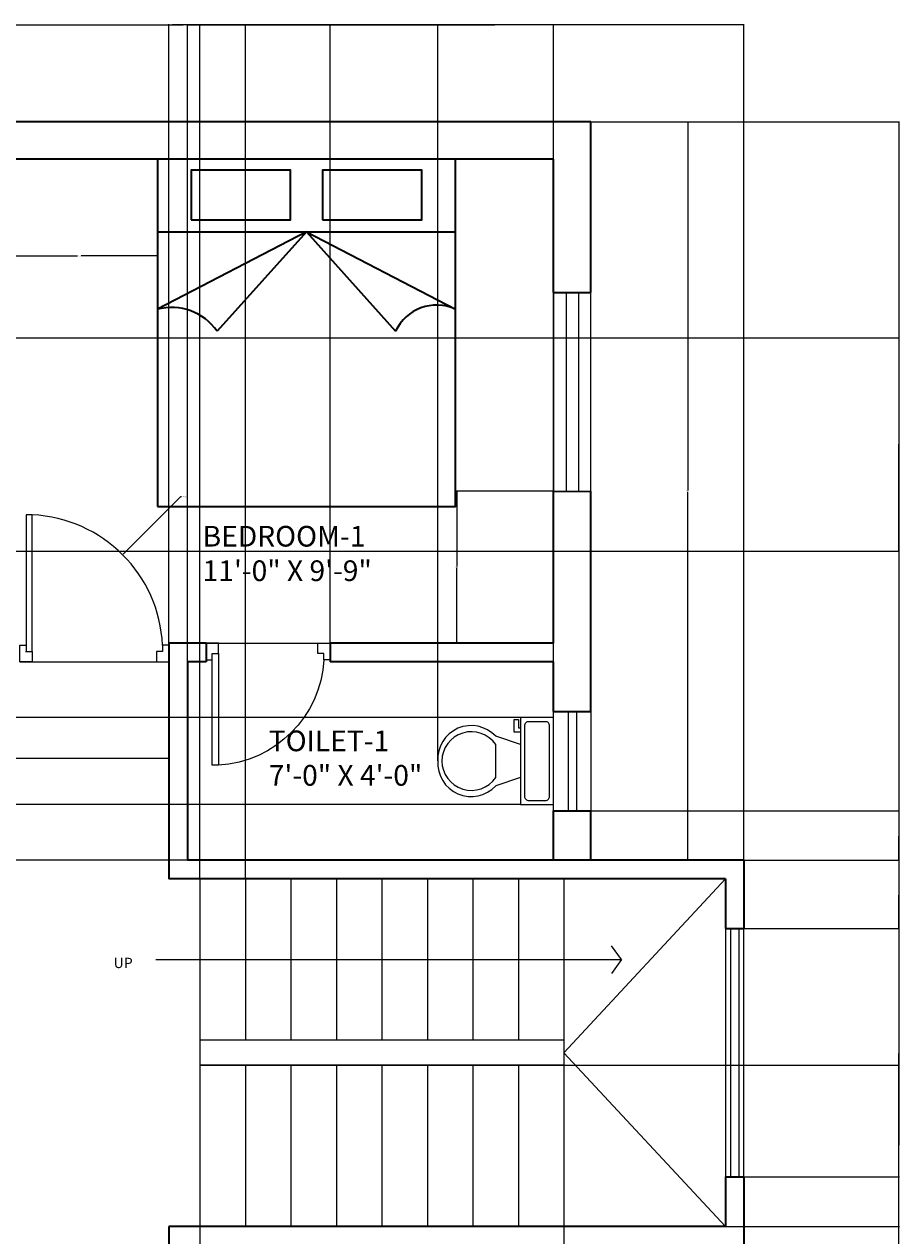
# Model space of a CAD drawing. Units: inches. Extents: x 324 to 662, y 102 to 605.
# Tile 4 of 4: x 451 to 662, y 313 to 605. Entities that reach past the tile are written whole.
import ezdxf

# ---------------------------------------------------------------- set-up
doc = ezdxf.new("R2010")
doc.units = ezdxf.units.IN
for name, color, linetype, lineweight in [('A-ANNO-DIMS', 2, 'Continuous', 18), ('A-ANNO-SYMB', 7, 'Continuous', 18), ('A-ANNO-TEXT', 7, 'Continuous', 18), ('A-AREA-IDEN', 7, 'Continuous', 25), ('A-FLOR-FIXT', 8, 'Continuous', 18), ('A-FLOR-STRS', 7, 'Continuous', 18), ('door', 82, 'Continuous', 25), ('furniture', 8, 'Continuous', 18), ('ventilator', 20, 'Continuous', 18), ('wall', 7, 'Continuous', 35), ('window', 50, 'Continuous', 18)]:
    doc.layers.add(name, color=color, linetype=linetype, lineweight=lineweight)
doc.styles.get("Standard").update_dxf_attribs({"font": 'arial.ttf'})
doc.dimstyles.get("Standard").update_dxf_attribs({"dimtxt": 0.18, "dimasz": 0.18, "dimexe": 0.18, "dimexo": 0.0625, "dimgap": 0.09, "dimtad": 0, "dimtih": 1, "dimtoh": 1, "dimdec": 4, "dimzin": 0, "dimdsep": 46, "dimtxsty": 'Standard', "dimcen": 0.09, "dimadec": 0, "dimazin": 0, "dimtfac": 1, "dimtdec": 4, "dimtofl": 0, "dimtmove": 0, "dimatfit": 3, "dimfxl": 1, "dimtolj": 1, "dimtzin": 0, "dimarcsym": 0})

# ---------------------------------------------------------------- blocks, each defined once
blk = doc.blocks.new('w1')
at = {"layer": 'window'}
for p, q in [((719.66, 290.3), (719.66, 242.3)), ((722.66, 290.3), (722.66, 242.3))]:
    blk.add_line(p, q, dxfattribs=at)
blk.add_lwpolyline([(716.66, 242.3), (725.66, 242.3), (725.66, 290.3), (716.66, 290.3)], close=True, dxfattribs=at)
blk = doc.blocks.new('v')
at = {"layer": 'ventilator'}
for p, q in [((1044.91, 377.37), (1044.91, 353.37)), ((1046.91, 377.37), (1046.91, 353.37))]:
    blk.add_line(p, q, dxfattribs=at)
blk.add_lwpolyline([(1041.41, 377.37), (1050.41, 377.37), (1050.41, 353.37), (1041.41, 353.37)], close=True, dxfattribs=at)
blk = doc.blocks.new('d1')
at = {"layer": 'door'}
blk.add_line((825.6, 316.36), (861.6, 316.36), dxfattribs=at)
blk.add_lwpolyline([(827.1, 318.86), (828.6, 318.86), (828.6, 351.86), (827.1, 351.86)], close=True, dxfattribs=at)
for points in [[(828.6, 316.36), (825.6, 316.36), (825.6, 320.36), (827.1, 320.36), (827.1, 318.86), (828.6, 318.86), (828.6, 316.36)], [(858.6, 316.36), (861.6, 316.36), (861.6, 320.36), (860.1, 320.36), (860.1, 318.86), (858.6, 318.86), (858.6, 316.36)]]:
    blk.add_lwpolyline(points, dxfattribs=at)
blk.add_arc((827.1, 318.86), 33.03, 2.6026, 87.3974, dxfattribs=at)
blk = doc.blocks.new('d2')
at = {"layer": 'door'}
blk.add_line((825.6, 261.67), (855.6, 261.67), dxfattribs=at)
blk.add_lwpolyline([(827.1, 264.17), (828.6, 264.17), (828.6, 291.17), (827.1, 291.17)], close=True, dxfattribs=at)
for points in [[(828.6, 261.67), (825.6, 261.67), (825.6, 265.67), (827.1, 265.67), (827.1, 264.17), (828.6, 264.17), (828.6, 261.67)], [(852.6, 261.67), (855.6, 261.67), (855.6, 265.67), (854.1, 265.67), (854.1, 264.17), (852.6, 264.17), (852.6, 261.67)]]:
    blk.add_lwpolyline(points, dxfattribs=at)
blk.add_arc((827.1, 264.17), 27.04, 3.1798, 86.8202, dxfattribs=at)
blk = doc.blocks.new('BED')
at = {"layer": 'wall'}
for p, q in [((215.01, 591.25), (287.01, 591.25)), ((251.01, 591.25), (215.01, 572.55)), ((251.01, 591.25), (229.44, 567.26)), ((251.01, 591.25), (287.01, 572.55)), ((251.01, 591.25), (272.58, 567.26))]:
    blk.add_line(p, q, dxfattribs=at)
for points in [[(215.01, 524.86), (287.01, 524.86), (287.01, 608.86), (215.01, 608.86)], [(223.15, 594.21), (247.15, 594.21), (247.15, 606.21), (223.15, 606.21)], [(254.93, 594.21), (278.93, 594.21), (278.93, 606.21), (254.93, 606.21)]]:
    blk.add_lwpolyline(points, close=True, dxfattribs=at)
for centre, radius, start, end in [((218.46, 559.65), 13.35, 34.7262, 104.9976), ((282.46, 562.63), 10.92, 65.3787, 154.8976)]:
    blk.add_arc(centre, radius, start, end, dxfattribs=at)
blk = doc.blocks.new('*U8')
for p, q in [((9.5, -6), (9.5, -2)), ((-10, -8.5), (-8, -8.5)), ((-10, -9.5), (-10, -8.5)), ((-8, -8.5), (-8, -8)), ((-7, -8), (-7, -9.5)), ((-4, -8), (-6, -14)), ((4, -8), (6, -14)), ((-7, -9.5), (-10, -9.5)), ((4, -14), (-4, -14))]:
    blk.add_line(p, q)
blk.add_lwpolyline([(10.5, -8), (10.5, 0), (-10.5, 0), (-10.5, -8)], close=True)
for points in [[(-9.5, -2), (-9.5, -6)], [(8.5, -1), (-8.5, -1)], [(-8.5, -7), (8.5, -7)]]:
    blk.add_lwpolyline(points)
for centre, radius, start, end in [((-8.625, -1.875), 0.8839, 81.8699, 188.1301), ((8.625, -1.875), 0.8839, 351.8699, 98.1301), ((-8.625, -6.125), 0.8839, 171.869898, 278.1301), ((8.625, -6.125), 0.8839, 261.8699, 8.1301), ((-0.4772, -19.9188), 8.0953, 133.01722, 273.38), ((0.0374, -19.8731), 7.127, 124.50543, 269.7), ((-0.0373, -19.8731), 7.127, 270.3, 55.4946), ((0.4773, -19.9188), 8.0953, 266.62, 46.9828)]:
    blk.add_arc(centre, radius, start, end)
blk = doc.blocks.new('*D24')
at = {"layer": 'A-ANNO-DIMS', "color": 0, "lineweight": -2, "transparency": 16777216}
for p, q in [((347.83, 581.92), (347.83, 605.45)), ((348.01, 605.27), (486.04, 605.27)), ((624.65, 605.27), (486.62, 605.27)), ((624.83, 403.42), (624.83, 605.45))]:
    blk.add_line(p, q, dxfattribs=at)
at = {"layer": 'A-ANNO-DIMS', "color": 0, "transparency": 16777216}
for points in [[(348.01, 605.3), (348.01, 605.24), (347.83, 605.27)], [(624.65, 605.3), (624.65, 605.24), (624.83, 605.27)]]:
    blk.add_solid(points, dxfattribs=at)
at = {"layer": 'Defpoints', "color": 0, "transparency": 16777216}
for p in [(624.83, 605.27), (347.83, 581.86), (624.83, 403.36)]:
    blk.add_point(p, dxfattribs=at)
at = {"layer": 'A-ANNO-DIMS', "color": 0, "transparency": 16777216, "insert": (486.33, 605.27), "char_height": 0.18, "attachment_point": 5}
blk.add_mtext('\\A1;277', dxfattribs=at)
blk = doc.blocks.new('*D25')
at = {"layer": 'A-ANNO-DIMS', "color": 0, "lineweight": -2, "transparency": 16777216}
for p, q in [((587.89, 581.86), (662.43, 581.86)), ((662.25, 581.68), (662.25, 354.04)), ((662.25, 126.04), (662.25, 353.68)), ((587.89, 125.86), (662.43, 125.86))]:
    blk.add_line(p, q, dxfattribs=at)
at = {"layer": 'A-ANNO-DIMS', "color": 0, "transparency": 16777216}
for points in [[(662.22, 581.68), (662.28, 581.68), (662.25, 581.86)], [(662.22, 126.04), (662.28, 126.04), (662.25, 125.86)]]:
    blk.add_solid(points, dxfattribs=at)
at = {"layer": 'Defpoints', "color": 0, "transparency": 16777216}
for p in [(587.83, 581.86), (587.83, 125.86), (662.25, 125.86)]:
    blk.add_point(p, dxfattribs=at)
at = {"layer": 'A-ANNO-DIMS', "color": 0, "transparency": 16777216, "insert": (662.25, 353.86), "char_height": 0.18, "attachment_point": 5}
blk.add_mtext('\\A1;456', dxfattribs=at)
blk = doc.blocks.new('*D32')
at = {"layer": 'A-ANNO-DIMS', "color": 0, "lineweight": -2, "transparency": 16777216}
for p, q in [((578.77, 492.61), (555.24, 492.61)), ((555.42, 492.43), (555.42, 474.42)), ((555.42, 456.04), (555.42, 474.05)), ((578.77, 455.86), (555.24, 455.86))]:
    blk.add_line(p, q, dxfattribs=at)
at = {"layer": 'A-ANNO-DIMS', "color": 0, "transparency": 16777216}
for points in [[(555.39, 492.43), (555.45, 492.43), (555.42, 492.61)], [(555.39, 456.04), (555.45, 456.04), (555.42, 455.86)]]:
    blk.add_solid(points, dxfattribs=at)
at = {"layer": 'Defpoints', "color": 0, "transparency": 16777216}
for p in [(555.42, 492.61), (578.83, 492.61), (578.83, 455.86)]:
    blk.add_point(p, dxfattribs=at)
at = {"layer": 'A-ANNO-DIMS', "color": 0, "transparency": 16777216, "insert": (555.42, 474.23), "char_height": 0.18, "attachment_point": 5}
blk.add_mtext('\\A1;36.75', dxfattribs=at)
blk = doc.blocks.new('*D33')
at = {"layer": 'A-ANNO-DIMS', "color": 0, "lineweight": -2, "transparency": 16777216}
for p, q in [((587.89, 415.36), (662.43, 415.36)), ((662.25, 415.18), (662.25, 409.54)), ((662.25, 403.54), (662.25, 409.18)), ((587.89, 403.36), (662.43, 403.36))]:
    blk.add_line(p, q, dxfattribs=at)
at = {"layer": 'A-ANNO-DIMS', "color": 0, "transparency": 16777216}
for points in [[(662.22, 415.18), (662.28, 415.18), (662.25, 415.36)], [(662.22, 403.54), (662.28, 403.54), (662.25, 403.36)]]:
    blk.add_solid(points, dxfattribs=at)
at = {"layer": 'Defpoints', "color": 0, "transparency": 16777216}
for p in [(587.83, 415.36), (587.83, 403.36), (662.25, 403.36)]:
    blk.add_point(p, dxfattribs=at)
at = {"layer": 'A-ANNO-DIMS', "color": 0, "transparency": 16777216, "insert": (662.25, 409.36), "char_height": 0.18, "attachment_point": 5}
blk.add_mtext('\\A1;12', dxfattribs=at)
blk = doc.blocks.new('*D34')
at = {"layer": 'A-ANNO-DIMS', "color": 0, "lineweight": -2, "transparency": 16777216}
for p, q in [((490.27, 403.36), (324.24, 403.36)), ((324.42, 403.18), (324.42, 357.04)), ((324.42, 310.54), (324.42, 356.68)), ((490.27, 310.36), (324.24, 310.36))]:
    blk.add_line(p, q, dxfattribs=at)
at = {"layer": 'A-ANNO-DIMS', "color": 0, "transparency": 16777216}
for points in [[(324.39, 403.18), (324.45, 403.18), (324.42, 403.36)], [(324.39, 310.54), (324.45, 310.54), (324.42, 310.36)]]:
    blk.add_solid(points, dxfattribs=at)
at = {"layer": 'Defpoints', "color": 0, "transparency": 16777216}
for p in [(490.33, 403.36), (324.42, 310.36), (490.33, 310.36)]:
    blk.add_point(p, dxfattribs=at)
at = {"layer": 'A-ANNO-DIMS', "color": 0, "transparency": 16777216, "insert": (324.42, 356.86), "char_height": 0.18, "attachment_point": 5}
blk.add_mtext('\\A1;93', dxfattribs=at)
blk = doc.blocks.new('*D35')
at = {"layer": 'A-ANNO-DIMS', "color": 0, "lineweight": -2, "transparency": 16777216}
for p, q in [((624.89, 386.86), (662.43, 386.86)), ((662.25, 386.68), (662.25, 357.04)), ((662.25, 327.04), (662.25, 356.68)), ((624.89, 326.86), (662.43, 326.86))]:
    blk.add_line(p, q, dxfattribs=at)
at = {"layer": 'A-ANNO-DIMS', "color": 0, "transparency": 16777216}
for points in [[(662.22, 386.68), (662.28, 386.68), (662.25, 386.86)], [(662.22, 327.04), (662.28, 327.04), (662.25, 326.86)]]:
    blk.add_solid(points, dxfattribs=at)
at = {"layer": 'Defpoints', "color": 0, "transparency": 16777216}
for p in [(624.83, 386.86), (624.83, 326.86), (662.25, 326.86)]:
    blk.add_point(p, dxfattribs=at)
at = {"layer": 'A-ANNO-DIMS', "color": 0, "transparency": 16777216, "insert": (662.25, 356.86), "char_height": 0.18, "attachment_point": 5}
blk.add_mtext('\\A1;60', dxfattribs=at)
blk = doc.blocks.new('*D36')
at = {"layer": 'A-ANNO-DIMS', "color": 0, "lineweight": -2, "transparency": 16777216}
for p, q in [((624.89, 403.36), (662.43, 403.36)), ((662.25, 403.18), (662.25, 395.29)), ((662.25, 387.04), (662.25, 394.93)), ((624.89, 386.86), (662.43, 386.86))]:
    blk.add_line(p, q, dxfattribs=at)
at = {"layer": 'A-ANNO-DIMS', "color": 0, "transparency": 16777216}
for points in [[(662.22, 403.18), (662.28, 403.18), (662.25, 403.36)], [(662.22, 387.04), (662.28, 387.04), (662.25, 386.86)]]:
    blk.add_solid(points, dxfattribs=at)
at = {"layer": 'Defpoints', "color": 0, "transparency": 16777216}
for p in [(624.83, 403.36), (624.83, 386.86), (662.25, 386.86)]:
    blk.add_point(p, dxfattribs=at)
at = {"layer": 'A-ANNO-DIMS', "color": 0, "transparency": 16777216, "insert": (662.25, 395.11), "char_height": 0.18, "attachment_point": 5}
blk.add_mtext('\\A1;16.5', dxfattribs=at)
blk = doc.blocks.new('*D44')
at = {"layer": 'A-ANNO-DIMS', "color": 0, "lineweight": -2, "transparency": 16777216}
for p, q in [((493.33, 314.8), (493.33, 102.17)), ((581.33, 314.8), (581.33, 102.17)), ((493.51, 102.35), (537.11, 102.35)), ((581.15, 102.35), (537.55, 102.35))]:
    blk.add_line(p, q, dxfattribs=at)
at = {"layer": 'A-ANNO-DIMS', "color": 0, "transparency": 16777216}
for points in [[(493.51, 102.38), (493.51, 102.32), (493.33, 102.35)], [(581.15, 102.38), (581.15, 102.32), (581.33, 102.35)]]:
    blk.add_solid(points, dxfattribs=at)
at = {"layer": 'Defpoints', "color": 0, "transparency": 16777216}
for p in [(493.33, 314.86), (581.33, 314.86), (581.33, 102.35)]:
    blk.add_point(p, dxfattribs=at)
at = {"layer": 'A-ANNO-DIMS', "color": 0, "transparency": 16777216, "insert": (537.33, 102.35), "char_height": 0.18, "attachment_point": 5}
blk.add_mtext('\\A1;88', dxfattribs=at)
blk = doc.blocks.new('*D45')
at = {"layer": 'A-ANNO-DIMS', "color": 0, "lineweight": -2, "transparency": 16777216}
for p, q in [((493.39, 353.86), (662.43, 353.86)), ((662.25, 353.68), (662.25, 334.54)), ((662.25, 315.04), (662.25, 334.18)), ((493.39, 314.86), (662.43, 314.86))]:
    blk.add_line(p, q, dxfattribs=at)
at = {"layer": 'A-ANNO-DIMS', "color": 0, "transparency": 16777216}
for points in [[(662.22, 353.68), (662.28, 353.68), (662.25, 353.86)], [(662.22, 315.04), (662.28, 315.04), (662.25, 314.86)]]:
    blk.add_solid(points, dxfattribs=at)
at = {"layer": 'Defpoints', "color": 0, "transparency": 16777216}
for p in [(493.33, 353.86), (662.25, 353.86), (493.33, 314.86)]:
    blk.add_point(p, dxfattribs=at)
at = {"layer": 'A-ANNO-DIMS', "color": 0, "transparency": 16777216, "insert": (662.25, 334.36), "char_height": 0.18, "attachment_point": 5}
blk.add_mtext('\\A1;39', dxfattribs=at)
blk = doc.blocks.new('*D46')
at = {"layer": 'A-ANNO-DIMS', "color": 0, "lineweight": -2, "transparency": 16777216}
for p, q in [((493.33, 398.92), (493.33, 605.45)), ((493.51, 605.27), (498.64, 605.27)), ((504.15, 605.27), (499.02, 605.27)), ((504.33, 398.92), (504.33, 605.45))]:
    blk.add_line(p, q, dxfattribs=at)
at = {"layer": 'A-ANNO-DIMS', "color": 0, "transparency": 16777216}
for points in [[(493.51, 605.3), (493.51, 605.24), (493.33, 605.27)], [(504.15, 605.3), (504.15, 605.24), (504.33, 605.27)]]:
    blk.add_solid(points, dxfattribs=at)
at = {"layer": 'Defpoints', "color": 0, "transparency": 16777216}
for p in [(504.33, 605.27), (493.33, 398.86), (504.33, 398.86)]:
    blk.add_point(p, dxfattribs=at)
at = {"layer": 'A-ANNO-DIMS', "color": 0, "transparency": 16777216, "insert": (498.83, 605.27), "char_height": 0.18, "attachment_point": 5}
blk.add_mtext('\\A1;11', dxfattribs=at)
blk = doc.blocks.new('*D47')
at = {"layer": 'A-ANNO-DIMS', "color": 0, "lineweight": -2, "transparency": 16777216}
for p, q in [((485.83, 398.92), (485.83, 605.45)), ((486.01, 605.27), (489.33, 605.27)), ((493.15, 605.27), (489.83, 605.27)), ((493.33, 398.92), (493.33, 605.45))]:
    blk.add_line(p, q, dxfattribs=at)
at = {"layer": 'A-ANNO-DIMS', "color": 0, "transparency": 16777216}
for points in [[(486.01, 605.3), (486.01, 605.24), (485.83, 605.27)], [(493.15, 605.3), (493.15, 605.24), (493.33, 605.27)]]:
    blk.add_solid(points, dxfattribs=at)
at = {"layer": 'Defpoints', "color": 0, "transparency": 16777216}
for p in [(493.33, 605.27), (485.83, 398.86), (493.33, 398.86)]:
    blk.add_point(p, dxfattribs=at)
at = {"layer": 'A-ANNO-DIMS', "color": 0, "transparency": 16777216, "insert": (489.58, 605.27), "char_height": 0.18, "attachment_point": 5}
blk.add_mtext('\\A1;7.5', dxfattribs=at)
blk = doc.blocks.new('*D50')
at = {"layer": 'A-ANNO-DIMS', "color": 0, "lineweight": -2, "transparency": 16777216}
for p, q in [((445.33, 572.8), (445.33, 549.26)), ((483.08, 572.8), (483.08, 549.26)), ((445.51, 549.44), (463.74, 549.44)), ((482.9, 549.44), (464.67, 549.44))]:
    blk.add_line(p, q, dxfattribs=at)
at = {"layer": 'A-ANNO-DIMS', "color": 0, "transparency": 16777216}
for points in [[(445.51, 549.47), (445.51, 549.41), (445.33, 549.44)], [(482.9, 549.47), (482.9, 549.41), (483.08, 549.44)]]:
    blk.add_solid(points, dxfattribs=at)
at = {"layer": 'Defpoints', "color": 0, "transparency": 16777216}
for p in [(445.33, 572.86), (483.08, 572.86), (445.33, 549.44)]:
    blk.add_point(p, dxfattribs=at)
at = {"layer": 'A-ANNO-DIMS', "color": 0, "transparency": 16777216, "insert": (464.21, 549.44), "char_height": 0.18, "attachment_point": 5}
blk.add_mtext('\\A1;37.754', dxfattribs=at)
blk = doc.blocks.new('*D53')
at = {"layer": 'A-ANNO-DIMS', "color": 0, "lineweight": -2, "transparency": 16777216}
for p, q in [((524.83, 451.42), (524.83, 605.45)), ((525.01, 605.27), (551.61, 605.27)), ((578.65, 605.27), (552.05, 605.27)), ((578.83, 403.42), (578.83, 605.45))]:
    blk.add_line(p, q, dxfattribs=at)
at = {"layer": 'A-ANNO-DIMS', "color": 0, "transparency": 16777216}
for points in [[(525.01, 605.3), (525.01, 605.24), (524.83, 605.27)], [(578.65, 605.3), (578.65, 605.24), (578.83, 605.27)]]:
    blk.add_solid(points, dxfattribs=at)
at = {"layer": 'Defpoints', "color": 0, "transparency": 16777216}
for p in [(578.83, 605.27), (524.83, 451.36), (578.83, 403.36)]:
    blk.add_point(p, dxfattribs=at)
at = {"layer": 'A-ANNO-DIMS', "color": 0, "transparency": 16777216, "insert": (551.83, 605.27), "char_height": 0.18, "attachment_point": 5}
blk.add_mtext('\\A1;54', dxfattribs=at)
blk = doc.blocks.new('*D56')
at = {"layer": 'A-ANNO-DIMS', "color": 0, "lineweight": -2, "transparency": 16777216}
for p, q in [((550.83, 427.42), (550.83, 605.45)), ((551.01, 605.27), (564.61, 605.27)), ((578.65, 605.27), (565.05, 605.27)), ((578.83, 437.92), (578.83, 605.45))]:
    blk.add_line(p, q, dxfattribs=at)
at = {"layer": 'A-ANNO-DIMS', "color": 0, "transparency": 16777216}
for points in [[(551.01, 605.3), (551.01, 605.24), (550.83, 605.27)], [(578.65, 605.3), (578.65, 605.24), (578.83, 605.27)]]:
    blk.add_solid(points, dxfattribs=at)
at = {"layer": 'Defpoints', "color": 0, "transparency": 16777216}
for p in [(578.83, 605.27), (578.83, 437.86), (550.83, 427.36)]:
    blk.add_point(p, dxfattribs=at)
at = {"layer": 'A-ANNO-DIMS', "color": 0, "transparency": 16777216, "insert": (564.83, 605.27), "char_height": 0.18, "attachment_point": 5}
blk.add_mtext('\\A1;28', dxfattribs=at)
blk = doc.blocks.new('*D57')
at = {"layer": 'A-ANNO-DIMS', "color": 0, "lineweight": -2, "transparency": 16777216}
for p, q in [((570.77, 437.86), (324.24, 437.86)), ((324.42, 437.68), (324.42, 427.54)), ((324.42, 417.04), (324.42, 427.18)), ((570.77, 416.86), (324.24, 416.86))]:
    blk.add_line(p, q, dxfattribs=at)
at = {"layer": 'A-ANNO-DIMS', "color": 0, "transparency": 16777216}
for points in [[(324.39, 437.68), (324.45, 437.68), (324.42, 437.86)], [(324.39, 417.04), (324.45, 417.04), (324.42, 416.86)]]:
    blk.add_solid(points, dxfattribs=at)
at = {"layer": 'Defpoints', "color": 0, "transparency": 16777216}
for p in [(324.42, 437.86), (570.83, 437.86), (570.83, 416.86)]:
    blk.add_point(p, dxfattribs=at)
at = {"layer": 'A-ANNO-DIMS', "color": 0, "transparency": 16777216, "insert": (324.42, 427.36), "char_height": 0.18, "attachment_point": 5}
blk.add_mtext('\\A1;21', dxfattribs=at)
blk = doc.blocks.new('*D58')
at = {"layer": 'A-ANNO-DIMS', "color": 0, "lineweight": -2, "transparency": 16777216}
for p, q in [((490.33, 403.42), (490.33, 605.45)), ((490.51, 605.27), (534.26, 605.27)), ((578.65, 605.27), (534.9, 605.27)), ((578.83, 403.42), (578.83, 605.45))]:
    blk.add_line(p, q, dxfattribs=at)
at = {"layer": 'A-ANNO-DIMS', "color": 0, "transparency": 16777216}
for points in [[(490.51, 605.3), (490.51, 605.24), (490.33, 605.27)], [(578.65, 605.3), (578.65, 605.24), (578.83, 605.27)]]:
    blk.add_solid(points, dxfattribs=at)
at = {"layer": 'Defpoints', "color": 0, "transparency": 16777216}
for p in [(578.83, 605.27), (490.33, 403.36), (578.83, 403.36)]:
    blk.add_point(p, dxfattribs=at)
at = {"layer": 'A-ANNO-DIMS', "color": 0, "transparency": 16777216, "insert": (534.58, 605.27), "char_height": 0.18, "attachment_point": 5}
blk.add_mtext('\\A1;88.5', dxfattribs=at)
blk = doc.blocks.new('*D60')
at = {"layer": 'A-ANNO-DIMS', "color": 0, "lineweight": -2, "transparency": 16777216}
for p, q in [((376.3, 529.67), (662.43, 529.67)), ((662.25, 529.49), (662.25, 504.05)), ((662.25, 478.25), (662.25, 503.69)), ((376.3, 478.07), (662.43, 478.07))]:
    blk.add_line(p, q, dxfattribs=at)
at = {"layer": 'A-ANNO-DIMS', "color": 0, "transparency": 16777216}
for points in [[(662.22, 529.49), (662.28, 529.49), (662.25, 529.67)], [(662.22, 478.25), (662.28, 478.25), (662.25, 478.07)]]:
    blk.add_solid(points, dxfattribs=at)
at = {"layer": 'Defpoints', "color": 0, "transparency": 16777216}
for p in [(376.24, 529.67), (662.25, 529.67), (376.24, 478.07)]:
    blk.add_point(p, dxfattribs=at)
at = {"layer": 'A-ANNO-DIMS', "color": 0, "transparency": 16777216, "insert": (662.25, 503.87), "char_height": 0.18, "attachment_point": 5}
blk.add_mtext('\\A1;51.6', dxfattribs=at)
blk = doc.blocks.new('*D62')
at = {"layer": 'A-ANNO-DIMS', "color": 0, "lineweight": -2, "transparency": 16777216}
for p, q in [((356.83, 451.3), (356.83, 427.76)), ((485.83, 451.3), (485.83, 427.76)), ((357.01, 427.94), (421.05, 427.94)), ((485.65, 427.94), (421.61, 427.94))]:
    blk.add_line(p, q, dxfattribs=at)
at = {"layer": 'A-ANNO-DIMS', "color": 0, "transparency": 16777216}
for points in [[(357.01, 427.97), (357.01, 427.91), (356.83, 427.94)], [(485.65, 427.97), (485.65, 427.91), (485.83, 427.94)]]:
    blk.add_solid(points, dxfattribs=at)
at = {"layer": 'Defpoints', "color": 0, "transparency": 16777216}
for p in [(356.83, 451.36), (485.83, 451.36), (356.83, 427.94)]:
    blk.add_point(p, dxfattribs=at)
at = {"layer": 'A-ANNO-DIMS', "color": 0, "transparency": 16777216, "insert": (421.33, 427.94), "char_height": 0.18, "attachment_point": 5}
blk.add_mtext('\\A1;129', dxfattribs=at)
blk = doc.blocks.new('*D68')
at = {"layer": 'A-ANNO-DIMS', "color": 0, "lineweight": -2, "transparency": 16777216}
for p, q in [((587.89, 581.86), (611.43, 581.86)), ((611.25, 581.68), (611.25, 492.79)), ((611.25, 403.54), (611.25, 492.43)), ((587.89, 403.36), (611.43, 403.36))]:
    blk.add_line(p, q, dxfattribs=at)
at = {"layer": 'A-ANNO-DIMS', "color": 0, "transparency": 16777216}
for points in [[(611.22, 581.68), (611.28, 581.68), (611.25, 581.86)], [(611.22, 403.54), (611.28, 403.54), (611.25, 403.36)]]:
    blk.add_solid(points, dxfattribs=at)
at = {"layer": 'Defpoints', "color": 0, "transparency": 16777216}
for p in [(587.83, 581.86), (587.83, 403.36), (611.25, 403.36)]:
    blk.add_point(p, dxfattribs=at)
at = {"layer": 'A-ANNO-DIMS', "color": 0, "transparency": 16777216, "insert": (611.25, 492.61), "char_height": 0.18, "attachment_point": 5}
blk.add_mtext('\\A1;178.5', dxfattribs=at)
blk = doc.blocks.new('*D69')
at = {"layer": 'A-ANNO-DIMS', "color": 0, "lineweight": -2, "transparency": 16777216}
for p, q in [((488.7, 491.23), (474.82, 477.35)), ((488.88, 491.23), (488.7, 491.23)), ((451.33, 453.77), (451.33, 453.95)), ((451.24, 453.86), (451.42, 453.86))]:
    blk.add_line(p, q, dxfattribs=at)
at = {"layer": 'A-ANNO-DIMS', "color": 0, "transparency": 16777216}
blk.add_solid([(474.8, 477.37), (474.84, 477.32), (474.69, 477.22)], dxfattribs=at)
at = {"layer": 'Defpoints', "color": 0, "transparency": 16777216}
for p in [(474.69, 477.22), (451.33, 453.86)]:
    blk.add_point(p, dxfattribs=at)
at = {"layer": 'A-ANNO-DIMS', "color": 0, "transparency": 16777216, "insert": (489.63, 491.23), "char_height": 0.18, "attachment_point": 5}
blk.add_mtext('\\A1;2X R33.034', dxfattribs=at)

msp = doc.modelspace()

# ---------------------------------------------------------------- linework, layer by layer
at = {"layer": 'A-ANNO-SYMB'}
for p, q in [((595.2252, 379.3598), (592.7903, 382.7192)), ((482.7259, 379.3598), (595.2252, 379.3598)), ((595.2252, 379.3598), (592.7903, 376.0003))]:
    msp.add_line(p, q, dxfattribs=at)
at = {"layer": 'A-FLOR-STRS'}
for p, q in [((493.3304, 398.8598), (493.3304, 314.8598)), ((504.3304, 398.8598), (504.3304, 359.8598)), ((515.3304, 398.8598), (515.3304, 359.8598)), ((526.3304, 398.8598), (526.3304, 359.8598)), ((537.3304, 398.8598), (537.3304, 359.8598)), ((548.3304, 398.8598), (548.3304, 359.8598)), ((559.3304, 398.8598), (559.3304, 359.8598)), ((570.3304, 398.8598), (570.3304, 359.8598)), ((581.3304, 398.8598), (581.3304, 314.8598)), ((581.3304, 356.8598), (620.3304, 398.8598)), ((581.3304, 359.8598), (493.3304, 359.8598)), ((581.3304, 356.8598), (620.3304, 314.8598)), ((581.3304, 353.8598), (493.3304, 353.8598)), ((504.3304, 353.8598), (504.3304, 314.8598)), ((515.3304, 353.8598), (515.3304, 314.8598)), ((526.3304, 353.8598), (526.3304, 314.8598)), ((537.3304, 353.8598), (537.3304, 314.8598)), ((548.3304, 353.8598), (548.3304, 314.8598)), ((559.3304, 353.8598), (559.3304, 314.8598)), ((570.3304, 353.8598), (570.3304, 314.8598))]:
    msp.add_line(p, q, dxfattribs=at)
at = {"layer": 'wall'}
for p, q in [((587.8304, 581.8598), (428.3193, 581.8598)), ((587.8304, 540.6098), (587.8304, 581.8598)), ((578.8304, 572.8598), (445.3304, 572.8598)), ((578.8304, 540.6098), (578.8304, 572.8598)), ((578.8304, 540.6098), (587.8304, 540.6098)), ((578.8304, 492.5221), (587.8304, 492.6098)), ((578.8304, 455.8598), (578.8304, 492.5221)), ((587.8304, 439.3598), (587.8304, 492.6098)), ((485.8304, 455.8598), (485.8304, 451.3598)), ((494.8304, 455.8598), (485.8304, 455.8598)), ((494.8304, 455.8598), (494.8304, 451.3598)), ((578.8304, 455.8598), (524.8304, 455.8598)), ((524.8304, 455.8598), (524.8304, 451.3598)), ((485.8304, 451.3598), (485.8304, 398.8598)), ((490.3304, 451.3598), (490.3304, 403.3598)), ((494.8304, 451.3598), (490.3304, 451.3598)), ((578.8304, 451.3598), (524.8304, 451.3598)), ((578.8304, 439.3598), (578.8304, 451.3598)), ((578.8304, 439.3598), (587.8304, 439.3598)), ((578.8304, 403.3598), (578.8304, 415.3598)), ((578.8304, 415.3598), (587.8304, 415.3598)), ((587.8304, 403.3598), (587.8304, 415.3598)), ((624.8304, 403.3598), (490.3304, 403.3598)), ((624.8304, 403.3598), (624.8304, 386.8598)), ((620.3304, 398.8598), (485.8304, 398.8598)), ((620.3304, 398.8598), (620.3304, 386.8598)), ((620.3304, 386.8598), (624.8304, 386.8598)), ((620.3304, 326.8598), (624.8304, 326.8598)), ((620.3304, 326.8598), (620.3304, 314.8598)), ((624.8304, 326.8598), (624.8304, 310.3598)), ((620.3304, 314.8598), (485.8304, 314.8598)), ((485.8304, 314.8598), (485.8304, 296.8598))]:
    msp.add_line(p, q, dxfattribs=at)
at = {"layer": 'window'}
for p, q in [((621.5804, 386.8598), (621.5804, 326.8598)), ((623.5804, 386.8598), (623.5804, 326.8598))]:
    msp.add_line(p, q, dxfattribs=at)
msp.add_lwpolyline([(620.3304, 326.8598), (624.8304, 326.8598), (624.8304, 386.8598), (620.3304, 386.8598)], close=True, dxfattribs=at)

# ---------------------------------------------------------------- block references
at = {"layer": 'A-FLOR-FIXT', "rotation": 270}
msp.add_blockref('*U8', (578.8304, 427.3598), dxfattribs=at)
at = {"layer": 'door'}
msp.add_blockref('d1', (-375.7743, 135.0041), dxfattribs=at)
at = {"layer": 'door', "xscale": -1, "rotation": 180}
msp.add_blockref('d2', (-330.7743, 717.5286), dxfattribs=at)
at = {"layer": 'furniture'}
msp.add_blockref('BED', (268.0778, -35.996), dxfattribs=at)
at = {"layer": 'ventilator'}
msp.add_blockref('v', (-462.5774, 61.9865), dxfattribs=at)
at = {"layer": 'window'}
msp.add_blockref('w1', (-137.8269, 250.3052), dxfattribs=at)

# ---------------------------------------------------------------- texts
at = {"layer": 'A-ANNO-TEXT', "insert": (472.4966, 379.8142), "char_height": 2.5, "attachment_point": 1}
msp.add_mtext_dynamic_manual_height_columns('UP', width=8.061961, gutter_width=12.5, heights=[0], dxfattribs=at)
at = {"layer": 'A-AREA-IDEN', "char_height": 5, "attachment_point": 1}
for s, insert in [('BEDROOM-1\\P11\'-0" X 9\'-9"', (494.0122, 484.1967)), ('TOILET-1\\P7\'-0" X 4\'-0"', (510, 434.7331))]:
    msp.add_mtext_dynamic_manual_height_columns(s, width=50.156641, gutter_width=12.5, heights=[0], dxfattribs=dict(at, insert=insert))

# ---------------------------------------------------------------- dimensions: what is measured, and where the dimension line sits
at = {"layer": 'A-ANNO-DIMS'}
for base, p1, p2, override, picture, middle in [((624.8304, 605.2748), (347.8304, 581.8598), (624.8304, 403.3598), {"dimdec": 0, "dimlfac": 1, "dimrnd": 0, "dimzin": 0, "dimdsep": 46, "dimlunit": 2}, '*D24', (486.3304, 605.2748)), ((493.3304, 605.2748), (485.8304, 398.8598), (493.3304, 398.8598), {"dimdec": 1, "dimlfac": 1, "dimrnd": 0, "dimzin": 0, "dimdsep": 46, "dimlunit": 2}, '*D47', (489.5804, 605.2748)), ((578.8304, 605.2748), (490.3304, 403.3598), (578.8304, 403.3598), {"dimdec": 1, "dimlfac": 1, "dimrnd": 0, "dimzin": 0, "dimdsep": 46, "dimlunit": 2}, '*D58', (534.5804, 605.2748)), ((504.3304, 605.2748), (493.3304, 398.8598), (504.3304, 398.8598), {"dimdec": 0, "dimlfac": 1, "dimrnd": 0, "dimzin": 0, "dimdsep": 46, "dimlunit": 2}, '*D46', (498.8304, 605.2748)), ((578.8304, 605.2748), (524.8304, 451.3598), (578.8304, 403.3598), {"dimdec": 0, "dimlfac": 1, "dimrnd": 0, "dimzin": 0, "dimdsep": 46, "dimlunit": 2}, '*D53', (551.8304, 605.2748)), ((578.8304, 605.2748), (550.8304, 427.3597), (578.8304, 437.8598), {"dimdec": 0, "dimlfac": 1, "dimrnd": 0, "dimzin": 0, "dimdsep": 46, "dimlunit": 2}, '*D56', (564.8304, 605.2748)), ((581.3304, 102.3527), (493.3304, 314.8598), (581.3304, 314.8598), {"dimdec": 0, "dimlfac": 1, "dimrnd": 0, "dimzin": 0, "dimdsep": 46, "dimlunit": 2}, '*D44', (537.3304, 102.3527))]:
    dim = msp.add_linear_dim(base=base, p1=p1, p2=p2, dimstyle='Standard', override=override, dxfattribs=at)
    dim.commit()
    dim.dimension.update_dxf_attribs({"geometry": picture, "text_midpoint": middle})
for base, p1, p2, angle, override, picture, middle in [((662.2454, 125.8598), (587.8304, 581.8598), (587.8304, 125.8598), 90, {"dimdec": 0, "dimlfac": 1, "dimrnd": 0, "dimzin": 0, "dimdsep": 46, "dimlunit": 2}, '*D25', (662.2454, 353.8598)), ((611.2454, 403.3598), (587.8304, 581.8598), (587.8304, 403.3598), 270, {"dimdec": 1, "dimlfac": 1, "dimrnd": 0, "dimzin": 0, "dimdsep": 46, "dimlunit": 2}, '*D68', (611.2454, 492.6098)), ((445.3304, 549.4448), (483.0848, 572.8598), (445.3304, 572.8598), 180, {"dimdec": 3, "dimlfac": 1, "dimrnd": 0, "dimzin": 0, "dimdsep": 46, "dimlunit": 2}, '*D50', (464.2076, 549.4448)), ((662.2454, 529.67), (376.2379, 478.07), (376.2379, 529.67), 90, {"dimdec": 1, "dimlfac": 1, "dimrnd": 0, "dimzin": 0, "dimdsep": 46, "dimlunit": 2}, '*D60', (662.2454, 503.87)), ((555.4154, 492.6098), (578.8304, 455.8598), (578.8304, 492.6098), 90, {"dimdec": 2, "dimlfac": 1, "dimrnd": 0, "dimzin": 0, "dimdsep": 46, "dimlunit": 2}, '*D32', (555.4154, 474.2348)), ((356.8304, 427.9448), (485.8304, 451.3598), (356.8304, 451.3598), 180, {"dimdec": 0, "dimlfac": 1, "dimrnd": 0, "dimzin": 0, "dimdsep": 46, "dimlunit": 2}, '*D62', (421.3304, 427.9448)), ((324.4154, 437.8598), (570.8304, 416.8598), (570.8304, 437.8598), 90, {"dimdec": 0, "dimlfac": 1, "dimrnd": 0, "dimzin": 0, "dimdsep": 46, "dimlunit": 2}, '*D57', (324.4154, 427.3598)), ((662.2454, 403.3598), (587.8304, 415.3598), (587.8304, 403.3598), 90, {"dimdec": 0, "dimlfac": 1, "dimrnd": 0, "dimzin": 0, "dimdsep": 46, "dimlunit": 2}, '*D33', (662.2454, 409.3598)), ((324.4154, 310.3598), (490.3304, 403.3598), (490.3304, 310.3598), 90, {"dimdec": 0, "dimlfac": 1, "dimrnd": 0, "dimzin": 0, "dimdsep": 46, "dimlunit": 2}, '*D34', (324.4154, 356.8598)), ((662.2454, 386.8598), (624.8304, 403.3598), (624.8304, 386.8598), 90, {"dimdec": 1, "dimlfac": 1, "dimrnd": 0, "dimzin": 0, "dimdsep": 46, "dimlunit": 2}, '*D36', (662.2454, 395.1098)), ((662.2454, 326.8598), (624.8304, 386.8598), (624.8304, 326.8598), 90, {"dimdec": 0, "dimlfac": 1, "dimrnd": 0, "dimzin": 0, "dimdsep": 46, "dimlunit": 2}, '*D35', (662.2454, 356.8598)), ((662.2454, 353.8598), (493.3304, 314.8598), (493.3304, 353.8598), 90, {"dimdec": 0, "dimlfac": 1, "dimrnd": 0, "dimzin": 0, "dimdsep": 46, "dimlunit": 2}, '*D45', (662.2454, 334.3598))]:
    dim = msp.add_linear_dim(base=base, p1=p1, p2=p2, angle=angle, dimstyle='Standard', override=override, dxfattribs=at)
    dim.commit()
    dim.dimension.update_dxf_attribs({"geometry": picture, "text_midpoint": middle})
dim = msp.add_radius_dim(center=(451.3304, 453.8598), mpoint=(474.6892, 477.2182), text='2X <>', dimstyle='Standard', override={"dimdec": 3, "dimlfac": 1, "dimrnd": 0, "dimzin": 0, "dimdsep": 46, "dimlunit": 2}, dxfattribs=at)
dim.commit()
dim.dimension.update_dxf_attribs({"geometry": '*D69', "text_midpoint": (489.6288, 491.2332), "dimtype": 164})

doc.saveas('drawing.dxf')
